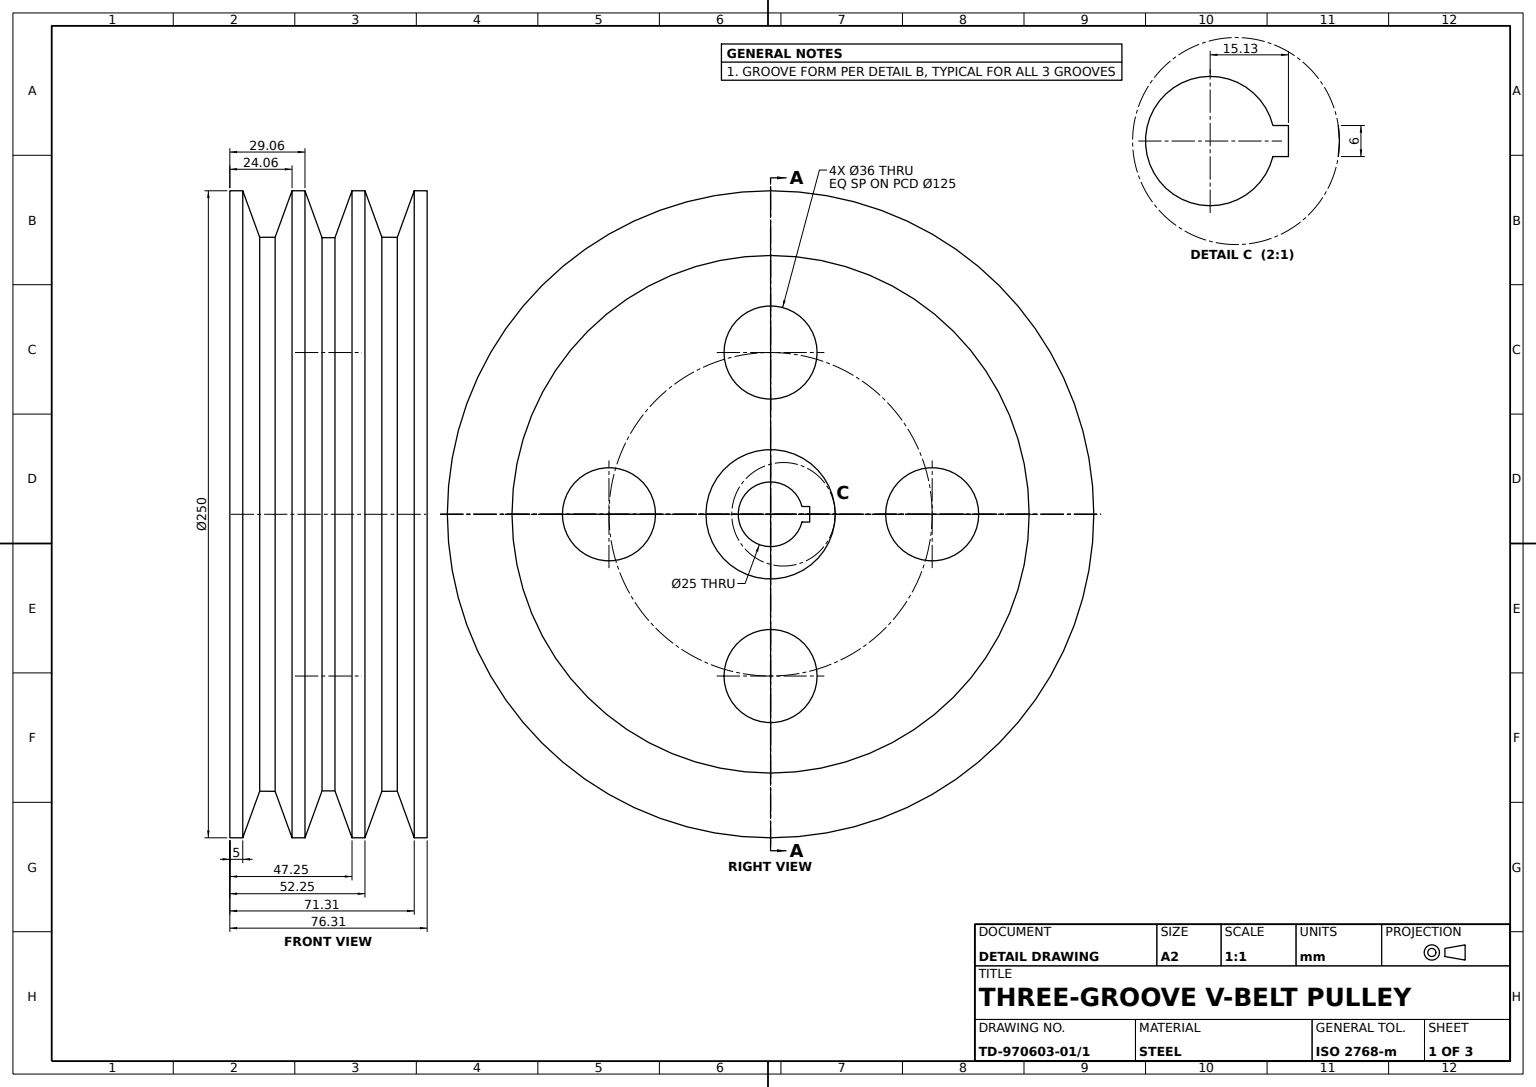
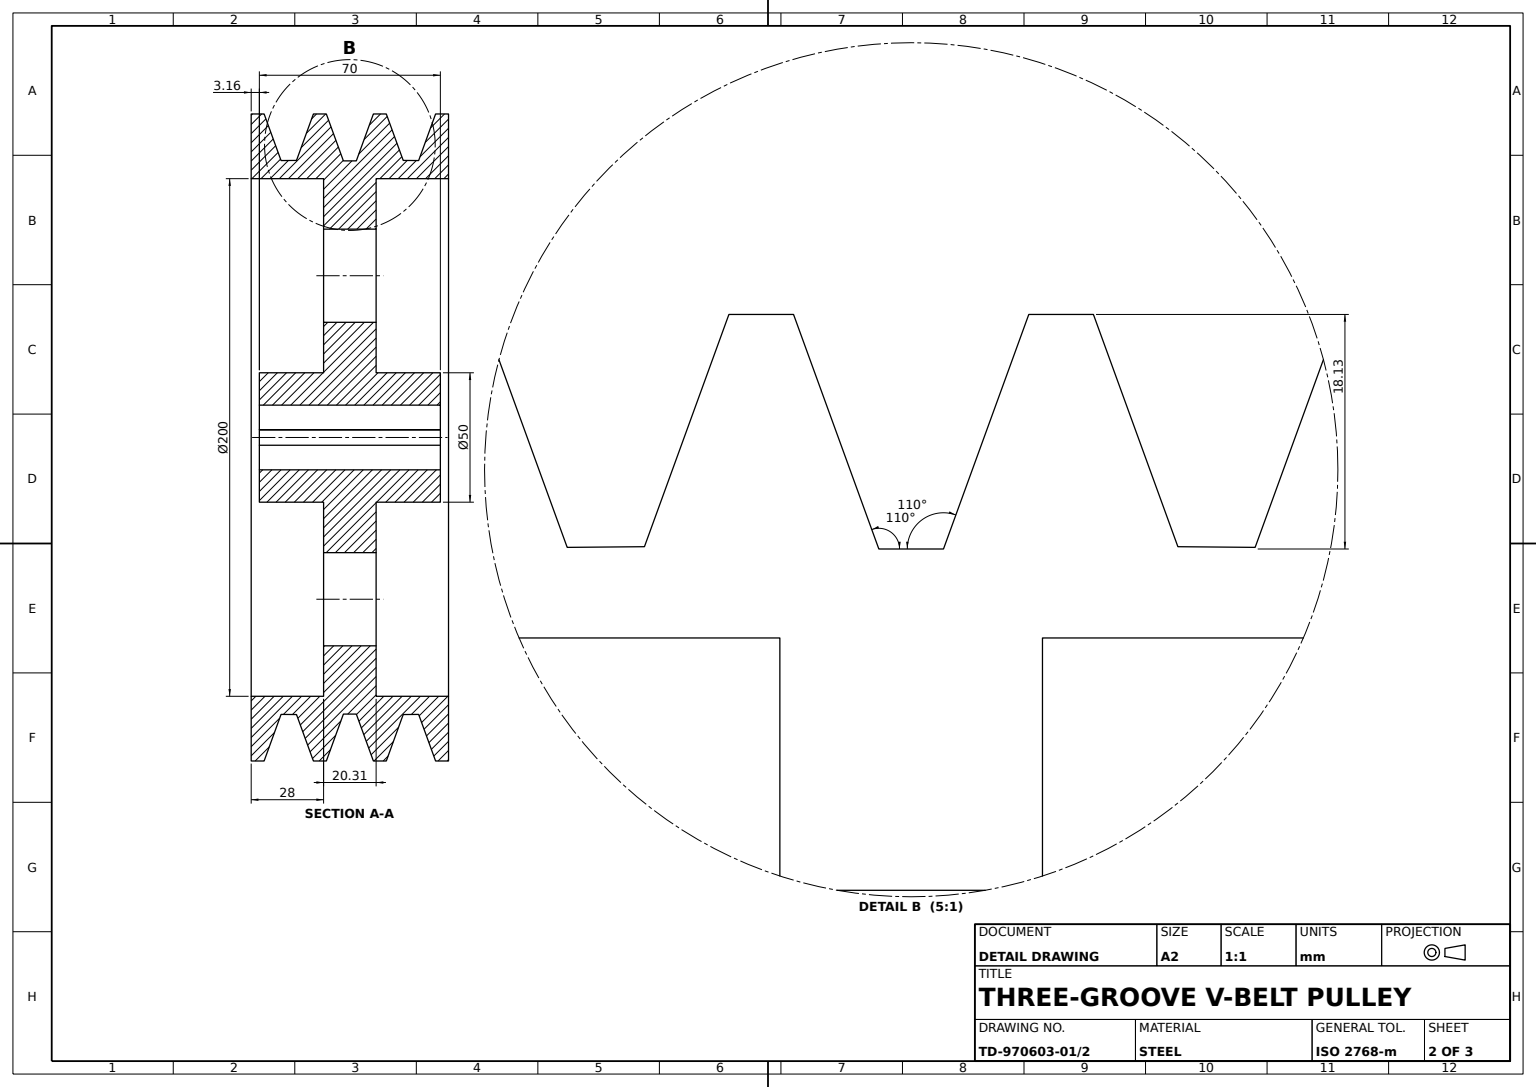
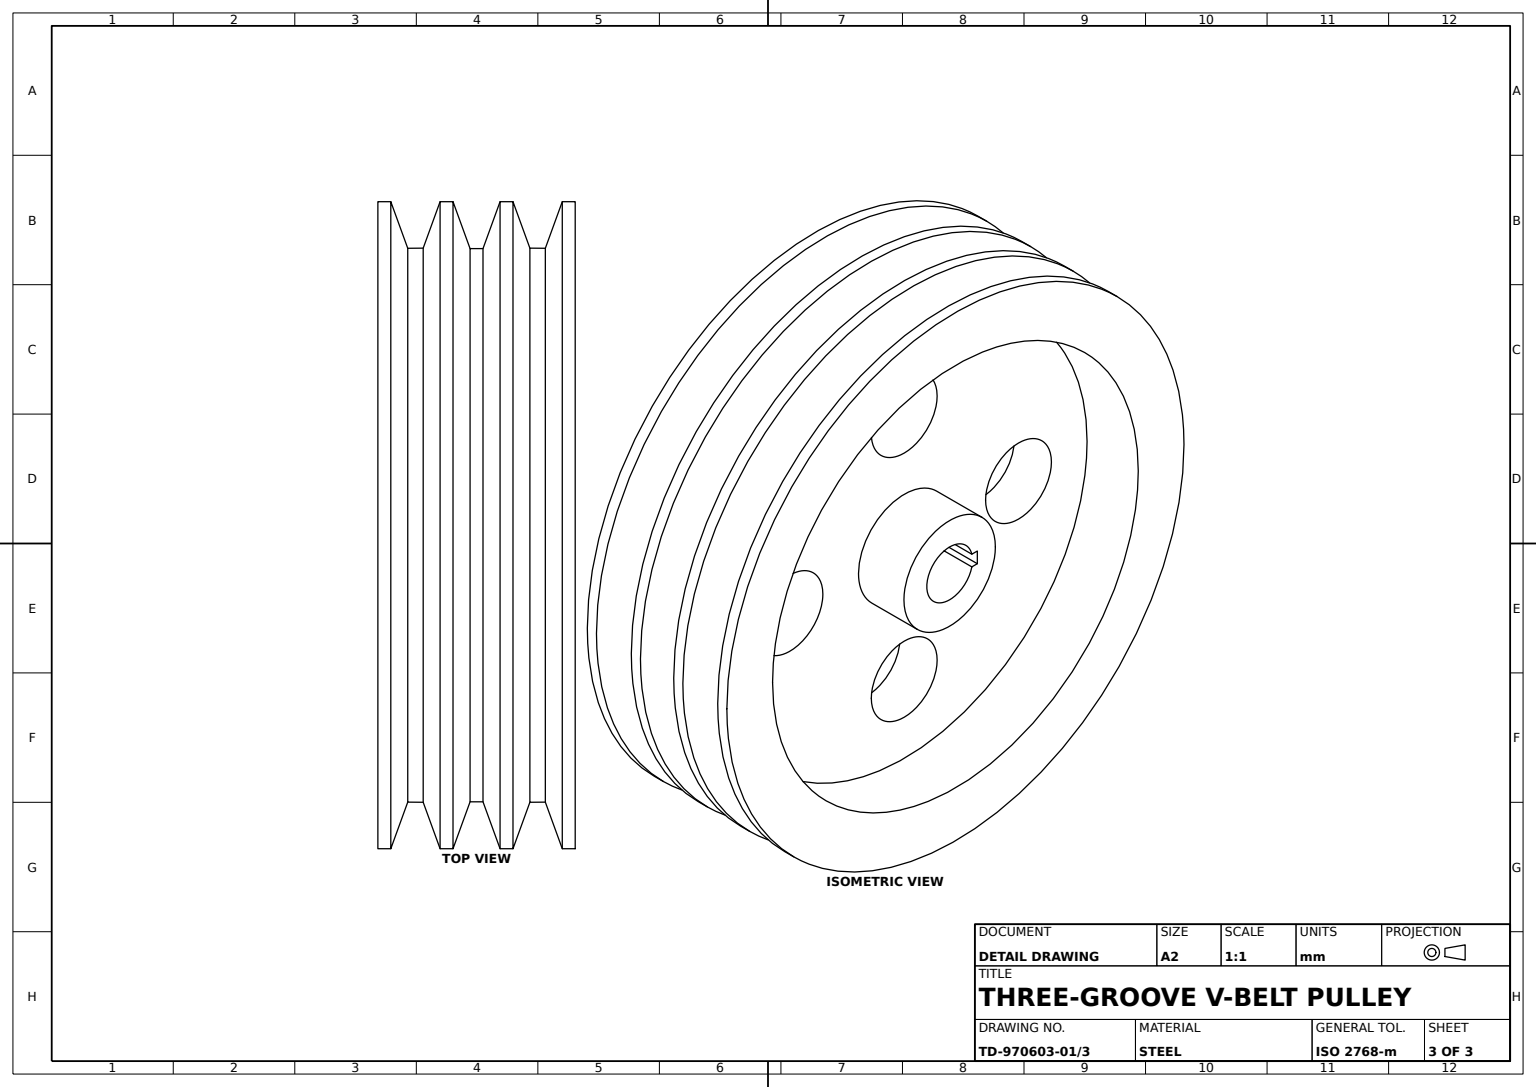
SolidWorks part; units mm, degrees
material "Plain Carbon Steel"
ref_plane "Front Plane" through (0, 0, 0) normal (0, 0, 1) x (1, 0, 0)
ref_plane "Top Plane" through (0, 0, 0) normal (0, 1, 0) x (1, 0, 0)
ref_plane "Right Plane" through (0, 0, 0) normal (1, 0, 0) x (0, 0, -1)
sketch "Pulley Profile Sketch" plane through (0, 0, 0) normal (0, 0, 1) x (1, 0, 0)
  line L0 (0, 145.2967) -> (0, -147.6614) construction
  line L1 (-177.5143, 0) -> (180.4104, 0) construction
  line L2 (-38.1556, 12.5) -> (38.1556, 12.5)
  line L3 (38.1556, 12.5) -> (38.1556, 125)
  line L5 (-38.1556, 12.5) -> (-38.1556, 125)
  line L6 (-38.1556, 125) -> (-33.1556, 125)
  line L8 (2.5, 106.8749) -> (9.097, 125)
  line L9 (-2.5, 106.8749) -> (-9.097, 125)
  line L10 (9.097, 125) -> (14.097, 125)
  line L11 (-14.097, 125) -> (-20.6292, 107.0528)
  line L12 (-20.6292, 107.0528) -> (-26.6042, 107)
  line L13 (-26.6042, 107) -> (-33.1556, 125)
  line L14 (-14.097, 125) -> (-9.097, 125)
  line L15 (20.6292, 107.0528) -> (26.6042, 107)
  line L16 (14.097, 125) -> (20.6292, 107.0528)
  line L17 (26.6042, 107) -> (33.1556, 125)
  line L18 (-2.5, 106.8749) -> (2.5, 106.8749)
  line L19 (33.1556, 125) -> (38.1556, 125)
  dimension "D1" = 12.5
  dimension "D2" = 5
  dimension "D3" = 40
  dimension "D4" = 9.097
  dimension "D5" = 18
  dimension "D6" = 5
  dimension "D7" = 14.097
  dimension "D8" = 20.6292
  dimension "D9" = 26.6042
  dimension "D10" = 125
revolve "Pulley Body 3-Groove" add sketch "Pulley Profile Sketch" angle 360 about L1
sketch "Web Recess Sketch" plane through (38.1556, 0, 0) normal (1, 0, 0) x (0, 0, -1)
  circle A0 centre (0, 0) radius 100
  dimension "D1" = 200
extrude "Web Recess Ø200" cut sketch "Web Recess Sketch" against normal blind 28
mirror "Web Recess Mirror" about plane through (0, 0, 0) normal (1, 0, 0) of "Web Recess Ø200"
sketch "Lightening Holes Sketch" plane through (0, 0, 0) normal (1, 0, 0) x (0, 0, -1)
  line L0 (0, 83.1785) -> (0, -87.1394) construction
  circle A0 centre (0, 0) radius 62.5 construction
  circle A1 centre (0, 62.5) radius 18
  circle A2 centre (62.5, 0) radius 18
  circle A3 centre (0, -62.5) radius 18
  circle A4 centre (-62.5, 0) radius 18
  point P16 (0, 0)
  dimension "D1" = 125
  dimension "D2" = 4
  dimension "D3" = 36
  dimension "D4" = 62.5
  dimension "D5" = 62.5
extrude "Lightening Holes 4x" cut sketch "Lightening Holes Sketch" against normal mid plane 22
sketch "Hub Sketch" plane through (0, 0, 0) normal (1, 0, 0) x (0, 0, -1)
  circle A0 centre (0, 0) radius 25
  dimension "D1" = 50
extrude "Hub Ø50" add sketch "Hub Sketch" along normal mid plane 70
sketch "Bore Sketch" plane through (0, 0, 0) normal (1, 0, 0) x (0, 0, -1)
  circle A0 centre (0, 0) radius 12.5
  dimension "D1" = 25
extrude "Bore Ø25" cut sketch "Bore Sketch" against normal mid plane 70
sketch "Keyway Sketch" plane through (0, 0, 0) normal (1, 0, 0) x (0, 0, -1)
  line L0 (12.1347, 3) -> (12.1347, -3)
  line L2 (15.1347, 3) -> (12.1347, 3)
  line L3 (15.1347, 3) -> (15.1347, -3)
  line L4 (15.1347, -3) -> (12.1347, -3)
  circle A0 centre (0, 0) radius 12.5 construction
  dimension "D1" = 3
  dimension "D2" = 6
  dimension "D3" = 3
extrude "Keyway 6x3" cut sketch "Keyway Sketch" against normal mid plane 70
